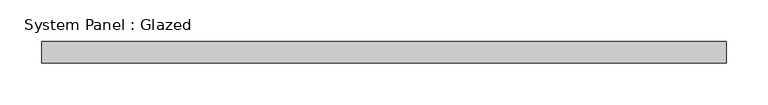
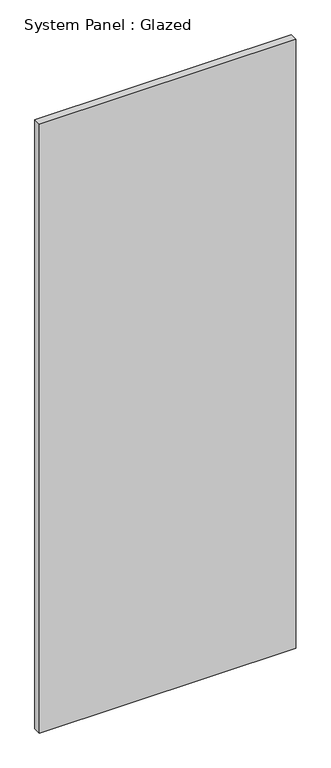
"""IFC4 building model written with IfcOpenShell, lengths in millimetres: plate geometry, System Panel : Glazed."""

from ifc_helpers import new_model, si_unit, origin, origin_with_axes, place, context, project, spatial, polyline, outline, extrude, source, transform, mapped, element, save


def system_panel_glazed_bec4471e(model_context):
    return source(origin(), model_context, "Body", "SweptSolid", [
        extrude(outline(polyline([(409.575, 19.05), (-409.575, 19.05), (-409.575, 44.45), (409.575, 44.45), (409.575, 19.05)])), origin_with_axes(), (0.0, 0.0, 1.0), 2057.4),
    ])


if __name__ == "__main__":
    model = new_model("IFC4")
    model_context = context("Model", 3, world=origin())
    ifc_project = project(units=[si_unit("LENGTHUNIT", "METRE", prefix="MILLI")], contexts=[model_context])
    site = spatial("IfcSite", under=ifc_project)
    building = spatial("IfcBuilding", under=site)
    placement = place(None, origin())
    system_panel_glazed_shape = system_panel_glazed_bec4471e(model_context)
    element("IfcPlate", 1, ObjectType="System Panel : Glazed", at=placement, inside=building, context=model_context, shape_type="MappedRepresentation", body=[
        mapped(system_panel_glazed_shape, transform((0.0, 0.0, 0.0), x_axis=(1.0, 0.0, 0.0), y_axis=(0.0, 1.0, 0.0), z_axis=(0.0, 0.0, 1.0))),
    ])
    save(model, "model.ifc")

# Revit data of these elements
# Type "System Panel : Glazed"
#   Construction Type Id = "GSP4R"
#   Analytic Construction = "1/8 in Pilkington single glazing"
#   Visual Light Transmittance = 0.9
#   Solar Heat Gain Coefficient = 0.86
#   Heat Transfer Coefficient (U) = 1.18115 BTU/(h·ft²·°F)
#   Define Thermal Properties by = 1
# Element 1 (IfcPlate, "System Panel : Glazed")
#   Materials on its faces: "Glass"
# Materials
#   "Glass": class "Glass", colour RGB 0 128 192, transparency 0.75, Description = "Soda Lime Glass", Cost = 0
